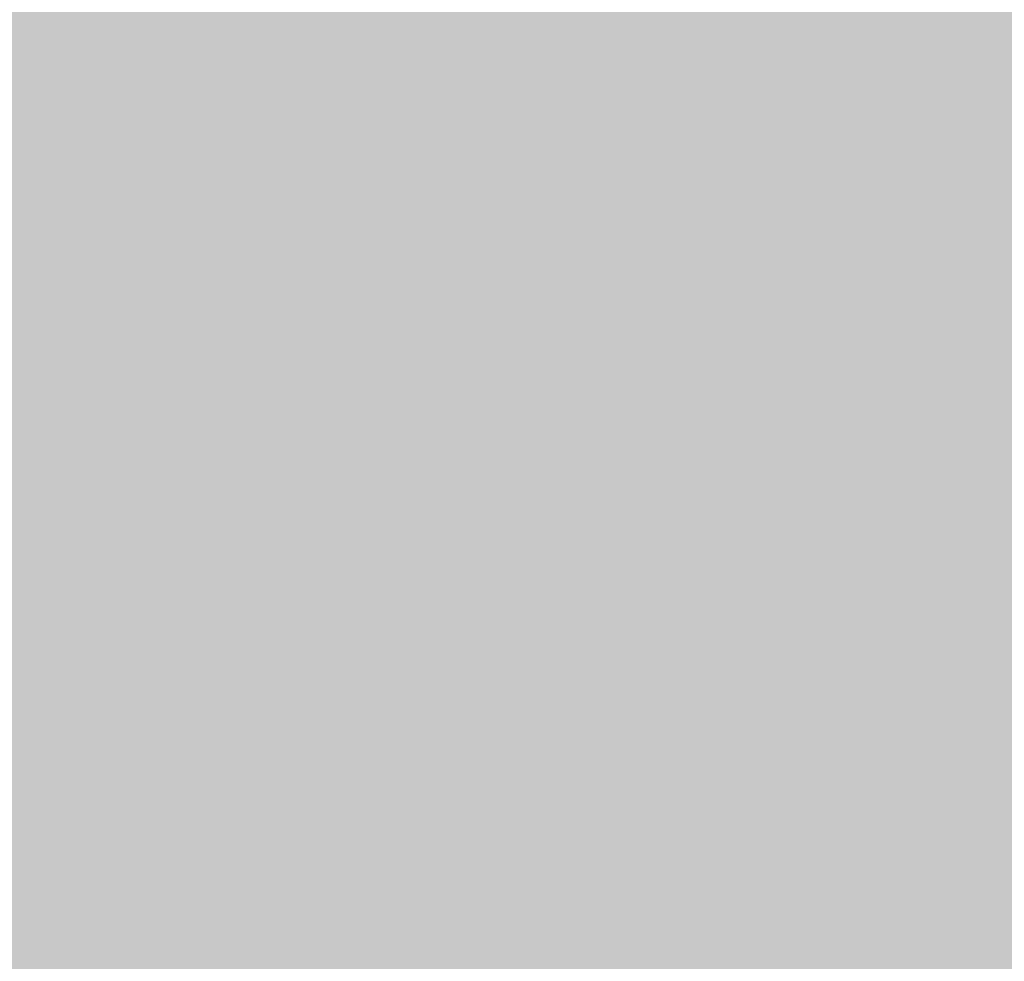
# Model space of a CAD drawing. Units: millimetres. Extents: x 0 to 2267, y 0 to 1823.
# Tile 202 of 256: x 1838.83 to 1841.442, y 1129.649 to 1132.147. Entities that reach past the tile are written whole.
import ezdxf

# ---------------------------------------------------------------- set-up
doc = ezdxf.new("R2010")
doc.units = ezdxf.units.MM
doc.header["$MEASUREMENT"] = 0
doc.layers.add('M-HATC', color=252, linetype='Continuous', lineweight=18)

msp = doc.modelspace()

# ---------------------------------------------------------------- hatches: boundary and pattern name
at = {"layer": 'M-HATC'}
h = msp.add_hatch(color=256, dxfattribs=at)
h.dxf.hatch_style = 1
h.paths.add_polyline_path([(2055.771, 1603.062), (1381.0868, 1603.062), (1381.0868, 1598.062), (2055.771, 1598.062)])
h.paths.add_polyline_path([(2055.771, 1598.062), (1381.0868, 1598.062), (1381.0868, 1593.062), (2055.771, 1593.062)])
h.paths.add_polyline_path([(2051.3074, 1536.7609), (1385.5504, 1536.7609), (1385.5504, 1526.7609), (1387.5504, 1526.7609), (1388.5366, 1525.0528), (1385.3319, 1521.2335), (1385.3319, 1521.2226), (2050.2542, 1522.7491), (2048.3212, 1525.0528), (2049.3074, 1526.7609), (2051.3074, 1526.7609)])
edge = h.paths.add_edge_path()
edge.add_arc((1847.5345, 1379.1492), 135, 222.603061, 222.890851, ccw=False)
edge.add_line((1748.1663, 1287.7656), (1683.0921, 1287.7656))
edge.add_arc((1583.7239, 1379.1492), 135, 317.109149, 317.396939, ccw=False)
edge.add_arc((1678.9686, 1290.6707), 5, 222.8909, 317.1091, ccw=False)
edge.add_arc((1774.2133, 1379.1492), 135, 222.603061, 222.890851, ccw=False)
edge.add_line((1674.8451, 1287.7656), (1609.7709, 1287.7656))
edge.add_arc((1510.4027, 1379.1492), 135, 317.109149, 317.396939, ccw=False)
edge.add_arc((1605.6474, 1290.6707), 5, 222.8909, 317.1091, ccw=False)
edge.add_arc((1700.8921, 1379.1492), 135, 222.603061, 222.890851, ccw=False)
edge.add_line((1601.5239, 1287.7656), (1536.4497, 1287.7656))
edge.add_arc((1437.0815, 1379.1492), 135, 317.109149, 317.396939, ccw=False)
edge.add_arc((1532.3262, 1290.6707), 5, 222.8909, 317.1091, ccw=False)
edge.add_arc((1627.5709, 1379.1492), 135, 222.603061, 222.890851, ccw=False)
edge.add_line((1528.2027, 1287.7656), (1505.9289, 1287.7656))
edge.add_spline(control_points=[(1505.9289, 1287.7656), (1504.2622, 1287.7656), (1504.2622, 1282.7656), (1505.9289, 1282.7656)], knot_values=[0, 0, 0, 0, 5, 5, 5, 5], degree=3, periodic=0)
edge.add_line((1505.9289, 1282.7656), (1930.9289, 1282.7656))
edge.add_spline(control_points=[(1930.9289, 1282.7656), (1932.5956, 1282.7656), (1932.5956, 1287.7656), (1930.9289, 1287.7656)], knot_values=[0, 0, 0, 0, 5, 5, 5, 5], degree=3, periodic=0)
edge.add_line((1930.9289, 1287.7656), (1903.0557, 1287.7656))
edge.add_arc((1803.6875, 1379.1492), 135, 317.109149, 317.396939, ccw=False)
edge.add_arc((1898.9322, 1290.6707), 5, 222.8909, 317.1091, ccw=False)
edge.add_arc((1994.1769, 1379.1492), 135, 222.603061, 222.890851, ccw=False)
edge.add_line((1894.8087, 1287.7656), (1829.7345, 1287.7656))
edge.add_arc((1730.3663, 1379.1492), 135, 317.109149, 317.396939, ccw=False)
edge.add_arc((1825.611, 1290.6707), 5, 222.8909, 317.1091, ccw=False)
edge.add_arc((1920.8557, 1379.1492), 135, 222.603061, 222.890851, ccw=False)
edge.add_line((1821.4875, 1287.7656), (1756.4133, 1287.7656))
edge.add_arc((1657.0451, 1379.1492), 135, 317.109149, 317.396939, ccw=False)
edge.add_arc((1752.2898, 1290.6707), 5, 222.8909, 317.1091, ccw=False)
edge = h.paths.add_edge_path()
edge.add_spline(control_points=[(1843.4289, 1227.2475), (1845.0956, 1227.2475), (1845.0956, 1232.2475), (1843.4289, 1232.2475)], knot_values=[0, 0, 0, 0, 5, 5, 5, 5], degree=3, periodic=0)
edge.add_line((1843.4289, 1232.2475), (1593.4289, 1232.2475))
edge.add_spline(control_points=[(1593.4289, 1232.2475), (1591.7622, 1232.2475), (1591.7622, 1227.2475), (1593.4289, 1227.2475)], knot_values=[0, 0, 0, 0, 5, 5, 5, 5], degree=3, periodic=0)
edge.add_line((1593.4289, 1227.2475), (1843.4289, 1227.2475))
h.paths.add_polyline_path([(1905.9289, 1127.4171), (1530.9289, 1127.4171, 0.414214), (1520.9289, 1117.4171), (1530.9289, 1117.4171), (1915.9289, 1117.4171, 0.414214)])
edge = h.paths.add_edge_path()
edge.add_arc((1397.0858, 1498.4078), 12.7299, 90.78215, 190.87871, ccw=False)
edge.add_line((1396.912, 1511.1365), (1428.0097, 1511.3488))
edge.add_line((1428.0097, 1511.3488), (1433.0097, 1511.3488))
edge.add_line((1433.0097, 1511.3488), (1434.439, 1511.3488))
edge.add_arc((1419.474, 1498.0804), 20, 41.561, 74.08211)
edge.add_line((1424.9592, 1517.3135), (1399.9351, 1517.2561))
edge.add_spline(control_points=[(1399.9307, 1517.2561), (1399.884, 1517.2131), (1399.8328, 1517.1689), (1399.7774, 1517.1236)], knot_values=[11.567499, 11.567499, 11.567499, 11.567499, 11.814249, 11.814249, 11.814249, 11.814249], degree=3, periodic=0)
edge.add_spline(control_points=[(1399.6328, 1517.0099), (1399.5831, 1516.9721), (1399.5307, 1516.9338), (1399.4759, 1516.8947)], knot_values=[11.167718, 11.167718, 11.167718, 11.167718, 11.365188, 11.365188, 11.365188, 11.365188], degree=3, periodic=0)
edge.add_spline(control_points=[(1399.3398, 1516.8001), (1399.1514, 1516.6719), (1398.9384, 1516.5377), (1398.704, 1516.3994)], knot_values=[10.376405, 10.376405, 10.376405, 10.376405, 11.00994, 11.00994, 11.00994, 11.00994], degree=3, periodic=0)
edge.add_spline(control_points=[(1398.6572, 1516.3719), (1398.5789, 1516.326), (1398.4983, 1516.2797), (1398.4155, 1516.2331)], knot_values=[10.125175, 10.125175, 10.125175, 10.125175, 10.334406, 10.334406, 10.334406, 10.334406], degree=3, periodic=0)
edge.add_spline(control_points=[(1398.2642, 1516.1487), (1398.196, 1516.1111), (1398.1263, 1516.0732), (1398.0555, 1516.0351)], knot_values=[9.832246, 9.832246, 9.832246, 9.832246, 9.999658, 9.999658, 9.999658, 9.999658], degree=3, periodic=0)
edge.add_spline(control_points=[(1397.9987, 1516.0048), (1397.7312, 1515.8621), (1397.446, 1515.7171), (1397.1466, 1515.5714)], knot_values=[9.161808, 9.161808, 9.161808, 9.161808, 9.787769, 9.787769, 9.787769, 9.787769], degree=3, periodic=0)
edge.add_spline(control_points=[(1397.1466, 1515.5714), (1396.8418, 1515.423), (1396.5222, 1515.274), (1396.1914, 1515.1262)], knot_values=[8.524455, 8.524455, 8.524455, 8.524455, 9.161808, 9.161808, 9.161808, 9.161808], degree=3, periodic=0)
edge.add_spline(control_points=[(1396.0777, 1515.0756), (1395.9854, 1515.0348), (1395.8922, 1514.994), (1395.7983, 1514.9534)], knot_values=[8.275193, 8.275193, 8.275193, 8.275193, 8.451726, 8.451726, 8.451726, 8.451726], degree=3, periodic=0)
edge.add_spline(control_points=[(1395.6018, 1514.8691), (1395.4997, 1514.8257), (1395.3968, 1514.7824), (1395.2932, 1514.7394)], knot_values=[7.962917, 7.962917, 7.962917, 7.962917, 8.152764, 8.152764, 8.152764, 8.152764], degree=3, periodic=0)
edge.add_spline(control_points=[(1395.2116, 1514.7057), (1394.8278, 1514.5475), (1394.4345, 1514.3929), (1394.0364, 1514.2442)], knot_values=[7.21254, 7.21254, 7.21254, 7.21254, 7.913148, 7.913148, 7.913148, 7.913148], degree=3, periodic=0)
edge.add_spline(control_points=[(1394.0364, 1514.2442), (1393.7076, 1514.1214), (1393.3754, 1514.0027), (1393.0427, 1513.8895)], knot_values=[6.633733, 6.633733, 6.633733, 6.633733, 7.21254, 7.21254, 7.21254, 7.21254], degree=3, periodic=0)
edge.add_spline(control_points=[(1392.8214, 1513.815), (1392.7198, 1513.7812), (1392.6181, 1513.7479), (1392.5166, 1513.7152)], knot_values=[6.328796, 6.328796, 6.328796, 6.328796, 6.505493, 6.505493, 6.505493, 6.505493], degree=3, periodic=0)
edge.add_spline(control_points=[(1392.5166, 1513.7152), (1392.3187, 1513.6515), (1392.1212, 1513.59), (1391.9244, 1513.531)], knot_values=[5.984605, 5.984605, 5.984605, 5.984605, 6.328796, 6.328796, 6.328796, 6.328796], degree=3, periodic=0)
edge.add_spline(control_points=[(1391.7915, 1513.4915), (1391.3122, 1513.3501), (1390.8384, 1513.2239), (1390.3784, 1513.1171)], knot_values=[5.066697, 5.066697, 5.066697, 5.066697, 5.907055, 5.907055, 5.907055, 5.907055], degree=3, periodic=0)
edge.add_spline(control_points=[(1390.3784, 1513.1171), (1390.1797, 1513.071), (1389.9836, 1513.0284), (1389.7907, 1512.9899)], knot_values=[4.70367, 4.70367, 4.70367, 4.70367, 5.066695, 5.066695, 5.066695, 5.066695], degree=3, periodic=0)
edge.add_spline(control_points=[(1389.422, 1512.9204), (1389.2459, 1512.8892), (1389.0729, 1512.8617), (1388.9036, 1512.8381)], knot_values=[4.130571, 4.130571, 4.130571, 4.130571, 4.469816, 4.469816, 4.469816, 4.469816], degree=3, periodic=0)
edge.add_spline(control_points=[(1388.9036, 1512.8381), (1388.591, 1512.7946), (1388.2911, 1512.7644), (1388.0071, 1512.7494)], knot_values=[3.504031, 3.504031, 3.504031, 3.504031, 4.130571, 4.130571, 4.130571, 4.130571], degree=3, periodic=0)
edge.add_spline(control_points=[(1387.9356, 1512.7459), (1387.8538, 1512.7423), (1387.7733, 1512.74), (1387.6944, 1512.739)], knot_values=[3.268866, 3.268866, 3.268866, 3.268866, 3.451164, 3.451164, 3.451164, 3.451164], degree=3, periodic=0)
edge.add_spline(control_points=[(1387.3351, 1512.7443), (1387.2076, 1512.7499), (1387.0847, 1512.7597), (1386.967, 1512.7739)], knot_values=[2.670686, 2.670686, 2.670686, 2.670686, 2.984, 2.984, 2.984, 2.984], degree=3, periodic=0)
edge.add_spline(control_points=[(1386.8327, 1512.7922), (1386.8209, 1512.7941), (1386.8092, 1512.7959), (1386.7975, 1512.7979)], knot_values=[2.516981, 2.516981, 2.516981, 2.516981, 2.549528, 2.549528, 2.549528, 2.549528], degree=3, periodic=0)
edge.add_spline(control_points=[(1386.4526, 1512.8735), (1386.4257, 1512.881), (1386.3993, 1512.889), (1386.3733, 1512.8972)], knot_values=[2.095869, 2.095869, 2.095869, 2.095869, 2.17941, 2.17941, 2.17941, 2.17941], degree=3, periodic=0)
edge.add_spline(control_points=[(1386.0691, 1513.0189), (1386.0634, 1513.0217), (1386.0577, 1513.0246), (1386.052, 1513.0275)], knot_values=[1.72453, 1.72453, 1.72453, 1.72453, 1.745933, 1.745933, 1.745933, 1.745933], degree=3, periodic=0)
edge.add_arc((1399.474, 1498.0804), 20, 131.82432, 180)
edge.add_arc((1630.3336, 1505.5484), 250.9708, 181.705176, 236.427975)
edge.add_arc((1605.3399, 1483.3044), 218.7822, 238.660829, 243.34961)
edge.add_arc((1647.0911, 1510.3592), 262.8986, 183.129836, 237.853442, ccw=False)
h.paths.add_polyline_path([(1406.5369, 1391.9644, 0.149382), (1491.5506, 1296.4418, -0.129517)], flags=17)
edge = h.paths.add_edge_path()
edge.add_arc((2037.3838, 1498.0804), 20, 0, 48.26587)
edge.add_spline(control_points=[(2050.6973, 1513.0052), (2050.6512, 1512.9847), (2050.6034, 1512.9655), (2050.5539, 1512.9477)], knot_values=[1.835652, 1.835652, 1.835652, 1.835652, 2.000781, 2.000781, 2.000781, 2.000781], degree=3, periodic=0)
edge.add_spline(control_points=[(2050.4616, 1512.9166), (2050.479, 1512.9221), (2050.4963, 1512.9277), (2050.5133, 1512.9335)], knot_values=[2.045477, 2.045477, 2.045477, 2.045477, 2.101389, 2.101389, 2.101389, 2.101389], degree=3, periodic=0)
edge.add_spline(control_points=[(2050.129, 1512.8342), (2050.1984, 1512.8473), (2050.2657, 1512.8623), (2050.3308, 1512.8792)], knot_values=[2.237629, 2.237629, 2.237629, 2.237629, 2.435841, 2.435841, 2.435841, 2.435841], degree=3, periodic=0)
edge.add_spline(control_points=[(2050.0946, 1512.8278), (2050.1061, 1512.8299), (2050.1176, 1512.832), (2050.129, 1512.8342)], knot_values=[2.435841, 2.435841, 2.435841, 2.435841, 2.468321, 2.468321, 2.468321, 2.468321], degree=3, periodic=0)
edge.add_spline(control_points=[(2049.7843, 1512.7851), (2049.8552, 1512.7922), (2049.9243, 1512.8008), (2049.9917, 1512.8109)], knot_values=[2.563852, 2.563852, 2.563852, 2.563852, 2.748541, 2.748541, 2.748541, 2.748541], degree=3, periodic=0)
edge.add_spline(control_points=[(2049.4052, 1512.7617), (2049.5364, 1512.7653), (2049.6629, 1512.773), (2049.7843, 1512.7851)], knot_values=[2.748541, 2.748541, 2.748541, 2.748541, 3.064882, 3.064882, 3.064882, 3.064882], degree=3, periodic=0)
edge.add_spline(control_points=[(2049.1698, 1512.7597), (2049.2336, 1512.7591), (2049.2965, 1512.7594), (2049.3584, 1512.7606)], knot_values=[3.102309, 3.102309, 3.102309, 3.102309, 3.2503, 3.2503, 3.2503, 3.2503], degree=3, periodic=0)
edge.add_spline(control_points=[(2048.8573, 1512.7691), (2048.9638, 1512.7638), (2049.068, 1512.7606), (2049.1698, 1512.7597)], knot_values=[3.2503, 3.2503, 3.2503, 3.2503, 3.486069, 3.486069, 3.486069, 3.486069], degree=3, periodic=0)
edge.add_spline(control_points=[(2048.6924, 1512.7789), (2048.3729, 1512.8009), (2048.0345, 1512.8411), (2047.6817, 1512.897)], knot_values=[3.606429, 3.606429, 3.606429, 3.606429, 4.2989, 4.2989, 4.2989, 4.2989], degree=3, periodic=0)
edge.add_spline(control_points=[(2047.6817, 1512.897), (2047.5458, 1512.9185), (2047.4077, 1512.9424), (2047.2678, 1512.9685)], knot_values=[4.2989, 4.2989, 4.2989, 4.2989, 4.565769, 4.565769, 4.565769, 4.565769], degree=3, periodic=0)
edge.add_spline(control_points=[(2047.2678, 1512.9685), (2047.1449, 1512.9914), (2047.0207, 1513.016), (2046.8951, 1513.0422)], knot_values=[4.565769, 4.565769, 4.565769, 4.565769, 4.799971, 4.799971, 4.799971, 4.799971], degree=3, periodic=0)
edge.add_spline(control_points=[(2046.8951, 1513.0422), (2046.5286, 1513.1188), (2046.1513, 1513.209), (2045.7676, 1513.3107)], knot_values=[4.799971, 4.799971, 4.799971, 4.799971, 5.483718, 5.483718, 5.483718, 5.483718], degree=3, periodic=0)
edge.add_spline(control_points=[(2045.7676, 1513.3107), (2045.3724, 1513.4154), (2044.9704, 1513.5322), (2044.5662, 1513.6588)], knot_values=[5.483718, 5.483718, 5.483718, 5.483718, 6.187866, 6.187866, 6.187866, 6.187866], degree=3, periodic=0)
edge.add_spline(control_points=[(2044.5662, 1513.6588), (2044.4149, 1513.7061), (2044.2633, 1513.7549), (2044.1116, 1513.8048)], knot_values=[6.187866, 6.187866, 6.187866, 6.187866, 6.451551, 6.451551, 6.451551, 6.451551], degree=3, periodic=0)
edge.add_spline(control_points=[(2044.1116, 1513.8048), (2043.9967, 1513.8427), (2043.8817, 1513.8813), (2043.7668, 1513.9205)], knot_values=[6.451551, 6.451551, 6.451551, 6.451551, 6.651434, 6.651434, 6.651434, 6.651434], degree=3, periodic=0)
edge.add_spline(control_points=[(2043.7668, 1513.9205), (2043.3716, 1514.0554), (2042.9774, 1514.1979), (2042.5886, 1514.3458)], knot_values=[6.651434, 6.651434, 6.651434, 6.651434, 7.338879, 7.338879, 7.338879, 7.338879], degree=3, periodic=0)
edge.add_spline(control_points=[(2042.5886, 1514.3458), (2042.1643, 1514.5071), (2041.7465, 1514.6749), (2041.3409, 1514.846)], knot_values=[7.338879, 7.338879, 7.338879, 7.338879, 8.089209, 8.089209, 8.089209, 8.089209], degree=3, periodic=0)
edge.add_spline(control_points=[(2041.3409, 1514.846), (2041.1028, 1514.9465), (2040.869, 1515.0481), (2040.6405, 1515.1502)], knot_values=[8.089209, 8.089209, 8.089209, 8.089209, 8.529587, 8.529587, 8.529587, 8.529587], degree=3, periodic=0)
edge.add_spline(control_points=[(2040.51, 1515.2089), (2040.0824, 1515.4022), (2039.6747, 1515.5971), (2039.295, 1515.7894)], knot_values=[8.613818, 8.613818, 8.613818, 8.613818, 9.44571, 9.44571, 9.44571, 9.44571], degree=3, periodic=0)
edge.add_spline(control_points=[(2039.295, 1515.7894), (2039.0618, 1515.9075), (2038.8391, 1516.0246), (2038.6288, 1516.1398)], knot_values=[9.44571, 9.44571, 9.44571, 9.44571, 9.956404, 9.956404, 9.956404, 9.956404], degree=3, periodic=0)
edge.add_spline(control_points=[(2038.6288, 1516.1398), (2038.5187, 1516.2001), (2038.4121, 1516.2598), (2038.309, 1516.3189)], knot_values=[9.956404, 9.956404, 9.956404, 9.956404, 10.223542, 10.223542, 10.223542, 10.223542], degree=3, periodic=0)
edge.add_spline(control_points=[(2038.309, 1516.3189), (2038.2138, 1516.3735), (2038.1216, 1516.4276), (2038.0328, 1516.481)], knot_values=[10.223542, 10.223542, 10.223542, 10.223542, 10.47051, 10.47051, 10.47051, 10.47051], degree=3, periodic=0)
edge.add_spline(control_points=[(2038.0328, 1516.481), (2037.7855, 1516.6296), (2037.5639, 1516.773), (2037.3722, 1516.909)], knot_values=[10.47051, 10.47051, 10.47051, 10.47051, 11.15767, 11.15767, 11.15767, 11.15767], degree=3, periodic=0)
edge.add_spline(control_points=[(2037.3722, 1516.909), (2037.2789, 1516.9752), (2037.1927, 1517.0396), (2037.1142, 1517.102)], knot_values=[11.15767, 11.15767, 11.15767, 11.15767, 11.49227, 11.49227, 11.49227, 11.49227], degree=3, periodic=0)
edge.add_spline(control_points=[(2036.8564, 1517.3259), (2036.9148, 1517.2692), (2036.9814, 1517.2103), (2037.0557, 1517.1492)], knot_values=[11.577341, 11.577341, 11.577341, 11.577341, 11.91035, 11.91035, 11.91035, 11.91035], degree=3, periodic=0)
edge.add_spline(control_points=[(2036.8074, 1517.3748), (2036.823, 1517.3587), (2036.8393, 1517.3424), (2036.8564, 1517.3259)], knot_values=[11.91035, 11.91035, 11.91035, 11.91035, 12.007402, 12.007402, 12.007402, 12.007402], degree=3, periodic=0)
edge.add_spline(control_points=[(2036.7017, 1517.494), (2036.7104, 1517.483), (2036.7196, 1517.4719), (2036.7291, 1517.4606)], knot_values=[12.184155, 12.184155, 12.184155, 12.184155, 12.255409, 12.255409, 12.255409, 12.255409], degree=3, periodic=0)
edge.add_spline(control_points=[(2036.6159, 1517.6205), (2036.62, 1517.613), (2036.6243, 1517.6055), (2036.6289, 1517.5979)], knot_values=[12.487913, 12.487913, 12.487913, 12.487913, 12.541035, 12.541035, 12.541035, 12.541035], degree=3, periodic=0)
edge.add_spline(control_points=[(2036.5635, 1517.786), (2036.5637, 1517.7794), (2036.5642, 1517.7726), (2036.565, 1517.7658)], knot_values=[12.911761, 12.911761, 12.911761, 12.911761, 12.968286, 12.968286, 12.968286, 12.968286], degree=3, periodic=0)
edge.add_spline(control_points=[(2036.6166, 1517.9304), (2036.6125, 1517.9259), (2036.6086, 1517.9212), (2036.6049, 1517.9165)], knot_values=[13.382527, 13.382527, 13.382527, 13.382527, 13.433791, 13.433791, 13.433791, 13.433791], degree=3, periodic=0)
edge.add_spline(control_points=[(2036.749, 1518.017), (2036.7361, 1518.0116), (2036.7239, 1518.006), (2036.7124, 1518.0002)], knot_values=[13.726299, 13.726299, 13.726299, 13.726299, 13.809928, 13.809928, 13.809928, 13.809928], degree=3, periodic=0)
edge.add_spline(control_points=[(2036.8604, 1518.0528), (2036.8386, 1518.0474), (2036.8181, 1518.0416), (2036.7988, 1518.0353)], knot_values=[13.910887, 13.910887, 13.910887, 13.910887, 14.02153, 14.02153, 14.02153, 14.02153], degree=3, periodic=0)
edge.add_line((2036.9639, 1518.0804), (2032.3838, 1518.0804))
edge.add_line((2032.3838, 1518.0804), (2027.3838, 1518.0804))
edge.add_line((2027.3838, 1518.0804), (2022.3838, 1518.0804))
edge.add_line((2022.3838, 1518.0804), (2017.3838, 1518.0804))
edge.add_arc((2017.3838, 1498.0804), 20, 90, 138.439)
edge.add_line((2002.4188, 1511.3488), (2003.8481, 1511.3488))
edge.add_line((2003.8481, 1511.3488), (2008.8481, 1511.3488))
edge.add_line((2008.8481, 1511.3488), (2039.772, 1511.1377))
edge.add_arc((2039.772, 1498.4078), 12.7299, -10.87871, 90, ccw=False)
edge.add_arc((1789.7668, 1510.3592), 262.8986, 302.146558, 356.870164, ccw=False)
edge.add_arc((1831.5179, 1483.3044), 218.7822, 296.65039, 301.339171)
edge.add_arc((1806.5242, 1505.5484), 250.9708, 303.572025, 358.294824)
h.paths.add_polyline_path([(2030.321, 1391.9644, -0.129517), (1945.3072, 1296.4418, 0.149382)], flags=17)
edge = h.paths.add_edge_path()
edge.add_spline(control_points=[(2037.2464, 1518.0821), (2037.2898, 1518.081), (2037.3355, 1518.0804), (2037.3838, 1518.0804)], knot_values=[0.000012, 0.000012, 0.000012, 0.000012, 0.144754, 0.144754, 0.144754, 0.144754], degree=3, periodic=0)
edge.add_line((2037.3357, 1518.0804), (2037.0096, 1518.0804))
edge.add_spline(control_points=[(2037.0096, 1518.0804), (2036.9822, 1518.0768), (2036.956, 1518.0727), (2036.9312, 1518.0681)], knot_values=[14.13465, 14.13465, 14.13465, 14.13465, 14.247197, 14.247197, 14.247197, 14.247197], degree=3, periodic=0)
edge.add_spline(control_points=[(2036.9312, 1518.0681), (2036.9276, 1518.0674), (2036.9241, 1518.0667), (2036.9205, 1518.0661)], knot_values=[14.118315, 14.118315, 14.118315, 14.118315, 14.13465, 14.13465, 14.13465, 14.13465], degree=3, periodic=0)
edge.add_spline(control_points=[(2036.9205, 1518.0661), (2036.9118, 1518.0644), (2036.9032, 1518.0626), (2036.8948, 1518.0608)], knot_values=[14.078086, 14.078086, 14.078086, 14.078086, 14.118315, 14.118315, 14.118315, 14.118315], degree=3, periodic=0)
edge.add_spline(control_points=[(2036.8948, 1518.0608), (2036.883, 1518.0583), (2036.8716, 1518.0556), (2036.8604, 1518.0528)], knot_values=[14.02153, 14.02153, 14.02153, 14.02153, 14.078086, 14.078086, 14.078086, 14.078086], degree=3, periodic=0)
edge.add_spline(control_points=[(2036.8604, 1518.0528), (2036.8386, 1518.0474), (2036.8181, 1518.0416), (2036.7988, 1518.0353)], knot_values=[13.910887, 13.910887, 13.910887, 13.910887, 14.02153, 14.02153, 14.02153, 14.02153], degree=3, periodic=0)
edge.add_spline(control_points=[(2036.7988, 1518.0353), (2036.7981, 1518.035), (2036.7974, 1518.0348), (2036.7967, 1518.0346)], knot_values=[13.906906, 13.906906, 13.906906, 13.906906, 13.910887, 13.910887, 13.910887, 13.910887], degree=3, periodic=0)
edge.add_spline(control_points=[(2036.7967, 1518.0346), (2036.7882, 1518.0318), (2036.7799, 1518.0289), (2036.7719, 1518.0259)], knot_values=[13.857826, 13.857826, 13.857826, 13.857826, 13.906906, 13.906906, 13.906906, 13.906906], degree=3, periodic=0)
edge.add_spline(control_points=[(2036.7719, 1518.0259), (2036.764, 1518.023), (2036.7564, 1518.02), (2036.749, 1518.017)], knot_values=[13.809928, 13.809928, 13.809928, 13.809928, 13.857826, 13.857826, 13.857826, 13.857826], degree=3, periodic=0)
edge.add_spline(control_points=[(2036.749, 1518.017), (2036.7361, 1518.0116), (2036.7239, 1518.006), (2036.7124, 1518.0002)], knot_values=[13.726299, 13.726299, 13.726299, 13.726299, 13.809928, 13.809928, 13.809928, 13.809928], degree=3, periodic=0)
edge.add_spline(control_points=[(2036.7124, 1518.0002), (2036.7121, 1518), (2036.7118, 1517.9999), (2036.7115, 1517.9997)], knot_values=[13.723993, 13.723993, 13.723993, 13.723993, 13.726299, 13.726299, 13.726299, 13.726299], degree=3, periodic=0)
edge.add_spline(control_points=[(2036.7115, 1517.9997), (2036.7063, 1517.9971), (2036.7013, 1517.9944), (2036.6965, 1517.9917)], knot_values=[13.686536, 13.686536, 13.686536, 13.686536, 13.723993, 13.723993, 13.723993, 13.723993], degree=3, periodic=0)
edge.add_spline(control_points=[(2036.6965, 1517.9917), (2036.6919, 1517.9891), (2036.6874, 1517.9865), (2036.6831, 1517.9839)], knot_values=[13.651251, 13.651251, 13.651251, 13.651251, 13.686536, 13.686536, 13.686536, 13.686536], degree=3, periodic=0)
edge.add_spline(control_points=[(2036.6831, 1517.9839), (2036.6764, 1517.9798), (2036.67, 1517.9757), (2036.6639, 1517.9714)], knot_values=[13.596804, 13.596804, 13.596804, 13.596804, 13.651251, 13.651251, 13.651251, 13.651251], degree=3, periodic=0)
edge.add_spline(control_points=[(2036.6639, 1517.9714), (2036.6636, 1517.9712), (2036.6633, 1517.9709), (2036.6629, 1517.9707)], knot_values=[13.593956, 13.593956, 13.593956, 13.593956, 13.596804, 13.596804, 13.596804, 13.596804], degree=3, periodic=0)
edge.add_spline(control_points=[(2036.6629, 1517.9707), (2036.6603, 1517.9689), (2036.6577, 1517.967), (2036.6552, 1517.9651)], knot_values=[13.570322, 13.570322, 13.570322, 13.570322, 13.593956, 13.593956, 13.593956, 13.593956], degree=3, periodic=0)
edge.add_spline(control_points=[(2036.6552, 1517.9651), (2036.6525, 1517.9631), (2036.6499, 1517.9611), (2036.6474, 1517.9591)], knot_values=[13.545477, 13.545477, 13.545477, 13.545477, 13.570322, 13.570322, 13.570322, 13.570322], degree=3, periodic=0)
edge.add_spline(control_points=[(2036.6474, 1517.9591), (2036.6472, 1517.9589), (2036.6471, 1517.9588), (2036.6469, 1517.9587)], knot_values=[13.543931, 13.543931, 13.543931, 13.543931, 13.545477, 13.545477, 13.545477, 13.545477], degree=3, periodic=0)
edge.add_spline(control_points=[(2036.6469, 1517.9587), (2036.6412, 1517.9541), (2036.6358, 1517.9494), (2036.6307, 1517.9447)], knot_values=[13.488237, 13.488237, 13.488237, 13.488237, 13.543931, 13.543931, 13.543931, 13.543931], degree=3, periodic=0)
edge.add_spline(control_points=[(2036.6307, 1517.9447), (2036.6282, 1517.9423), (2036.6257, 1517.9399), (2036.6233, 1517.9374)], knot_values=[13.460307, 13.460307, 13.460307, 13.460307, 13.488237, 13.488237, 13.488237, 13.488237], degree=3, periodic=0)
edge.add_spline(control_points=[(2036.6233, 1517.9374), (2036.6215, 1517.9356), (2036.6198, 1517.9338), (2036.6181, 1517.932)], knot_values=[13.439712, 13.439712, 13.439712, 13.439712, 13.460307, 13.460307, 13.460307, 13.460307], degree=3, periodic=0)
edge.add_spline(control_points=[(2036.6181, 1517.932), (2036.6176, 1517.9315), (2036.6171, 1517.9309), (2036.6166, 1517.9304)], knot_values=[13.433791, 13.433791, 13.433791, 13.433791, 13.439712, 13.439712, 13.439712, 13.439712], degree=3, periodic=0)
edge.add_spline(control_points=[(2036.6166, 1517.9304), (2036.6125, 1517.9259), (2036.6086, 1517.9212), (2036.6049, 1517.9165)], knot_values=[13.382527, 13.382527, 13.382527, 13.382527, 13.433791, 13.433791, 13.433791, 13.433791], degree=3, periodic=0)
edge.add_spline(control_points=[(2036.6049, 1517.9165), (2036.6026, 1517.9135), (2036.6004, 1517.9104), (2036.5982, 1517.9074)], knot_values=[13.350017, 13.350017, 13.350017, 13.350017, 13.382527, 13.382527, 13.382527, 13.382527], degree=3, periodic=0)
edge.add_spline(control_points=[(2036.5982, 1517.9074), (2036.5972, 1517.9059), (2036.5962, 1517.9043), (2036.5952, 1517.9028)], knot_values=[13.333922, 13.333922, 13.333922, 13.333922, 13.350017, 13.350017, 13.350017, 13.350017], degree=3, periodic=0)
edge.add_spline(control_points=[(2036.5952, 1517.9028), (2036.5945, 1517.9018), (2036.5939, 1517.9009), (2036.5933, 1517.8999)], knot_values=[13.323828, 13.323828, 13.323828, 13.323828, 13.333922, 13.333922, 13.333922, 13.333922], degree=3, periodic=0)
edge.add_spline(control_points=[(2036.5933, 1517.8999), (2036.5905, 1517.8955), (2036.5879, 1517.8909), (2036.5855, 1517.8864)], knot_values=[13.277545, 13.277545, 13.277545, 13.277545, 13.323828, 13.323828, 13.323828, 13.323828], degree=3, periodic=0)
edge.add_spline(control_points=[(2036.5855, 1517.8864), (2036.5836, 1517.8827), (2036.5817, 1517.8789), (2036.5801, 1517.8751)], knot_values=[13.240119, 13.240119, 13.240119, 13.240119, 13.277545, 13.277545, 13.277545, 13.277545], degree=3, periodic=0)
edge.add_spline(control_points=[(2036.5801, 1517.8751), (2036.5795, 1517.8739), (2036.579, 1517.8727), (2036.5785, 1517.8715)], knot_values=[13.228211, 13.228211, 13.228211, 13.228211, 13.240119, 13.240119, 13.240119, 13.240119], degree=3, periodic=0)
edge.add_spline(control_points=[(2036.5785, 1517.8715), (2036.578, 1517.8702), (2036.5774, 1517.869), (2036.5769, 1517.8677)], knot_values=[13.215717, 13.215717, 13.215717, 13.215717, 13.228211, 13.228211, 13.228211, 13.228211], degree=3, periodic=0)
edge.add_spline(control_points=[(2036.5769, 1517.8677), (2036.5755, 1517.864), (2036.5741, 1517.8603), (2036.5729, 1517.8565)], knot_values=[13.179847, 13.179847, 13.179847, 13.179847, 13.215717, 13.215717, 13.215717, 13.215717], degree=3, periodic=0)
edge.add_spline(control_points=[(2036.5729, 1517.8565), (2036.5713, 1517.8515), (2036.5699, 1517.8464), (2036.5687, 1517.8413)], knot_values=[13.132017, 13.132017, 13.132017, 13.132017, 13.179847, 13.179847, 13.179847, 13.179847], degree=3, periodic=0)
edge.add_spline(control_points=[(2036.5687, 1517.8413), (2036.5684, 1517.8402), (2036.5682, 1517.8392), (2036.568, 1517.8382)], knot_values=[13.122482, 13.122482, 13.122482, 13.122482, 13.132017, 13.132017, 13.132017, 13.132017], degree=3, periodic=0)
edge.add_spline(control_points=[(2036.568, 1517.8382), (2036.5676, 1517.8363), (2036.5672, 1517.8345), (2036.5669, 1517.8327)], knot_values=[13.105592, 13.105592, 13.105592, 13.105592, 13.122482, 13.122482, 13.122482, 13.122482], degree=3, periodic=0)
edge.add_spline(control_points=[(2036.5669, 1517.8327), (2036.5662, 1517.8292), (2036.5657, 1517.8257), (2036.5652, 1517.8222)], knot_values=[13.074063, 13.074063, 13.074063, 13.074063, 13.105592, 13.105592, 13.105592, 13.105592], degree=3, periodic=0)
edge.add_spline(control_points=[(2036.5652, 1517.8222), (2036.5652, 1517.8222), (2036.5652, 1517.8222), (2036.5652, 1517.8222)], knot_values=[13.074043, 13.074043, 13.074043, 13.074043, 13.074063, 13.074063, 13.074063, 13.074063], degree=3, periodic=0)
edge.add_spline(control_points=[(2036.5652, 1517.8222), (2036.5644, 1517.8164), (2036.5639, 1517.8106), (2036.5636, 1517.8046)], knot_values=[13.021884, 13.021884, 13.021884, 13.021884, 13.074043, 13.074043, 13.074043, 13.074043], degree=3, periodic=0)
edge.add_spline(control_points=[(2036.5636, 1517.8046), (2036.5636, 1517.804), (2036.5636, 1517.8034), (2036.5635, 1517.8028)], knot_values=[13.01674, 13.01674, 13.01674, 13.01674, 13.021884, 13.021884, 13.021884, 13.021884], degree=3, periodic=0)
edge.add_spline(control_points=[(2036.5635, 1517.8028), (2036.5634, 1517.8005), (2036.5634, 1517.7982), (2036.5634, 1517.7958)], knot_values=[12.996438, 12.996438, 12.996438, 12.996438, 13.01674, 13.01674, 13.01674, 13.01674], degree=3, periodic=0)
edge.add_spline(control_points=[(2036.5634, 1517.7958), (2036.5633, 1517.7926), (2036.5634, 1517.7893), (2036.5635, 1517.786)], knot_values=[12.968286, 12.968286, 12.968286, 12.968286, 12.996438, 12.996438, 12.996438, 12.996438], degree=3, periodic=0)
edge.add_spline(control_points=[(2036.5635, 1517.786), (2036.5637, 1517.7794), (2036.5642, 1517.7726), (2036.565, 1517.7658)], knot_values=[12.911761, 12.911761, 12.911761, 12.911761, 12.968286, 12.968286, 12.968286, 12.968286], degree=3, periodic=0)
edge.add_spline(control_points=[(2036.565, 1517.7658), (2036.565, 1517.7657), (2036.565, 1517.7656), (2036.565, 1517.7656)], knot_values=[12.911017, 12.911017, 12.911017, 12.911017, 12.911761, 12.911761, 12.911761, 12.911761], degree=3, periodic=0)
edge.add_spline(control_points=[(2036.565, 1517.7656), (2036.5654, 1517.7625), (2036.5658, 1517.7593), (2036.5663, 1517.7562)], knot_values=[12.88528, 12.88528, 12.88528, 12.88528, 12.911017, 12.911017, 12.911017, 12.911017], degree=3, periodic=0)
edge.add_spline(control_points=[(2036.5663, 1517.7562), (2036.5667, 1517.7534), (2036.5672, 1517.7506), (2036.5677, 1517.7478)], knot_values=[12.862519, 12.862519, 12.862519, 12.862519, 12.88528, 12.88528, 12.88528, 12.88528], degree=3, periodic=0)
edge.add_spline(control_points=[(2036.5677, 1517.7478), (2036.5678, 1517.7474), (2036.5679, 1517.7469), (2036.568, 1517.7465)], knot_values=[12.858885, 12.858885, 12.858885, 12.858885, 12.862519, 12.862519, 12.862519, 12.862519], degree=3, periodic=0)
edge.add_spline(control_points=[(2036.568, 1517.7465), (2036.5692, 1517.7399), (2036.5707, 1517.7332), (2036.5724, 1517.7264)], knot_values=[12.8053, 12.8053, 12.8053, 12.8053, 12.858885, 12.858885, 12.858885, 12.858885], degree=3, periodic=0)
edge.add_spline(control_points=[(2036.5724, 1517.7264), (2036.5734, 1517.7226), (2036.5745, 1517.7187), (2036.5756, 1517.7149)], knot_values=[12.775176, 12.775176, 12.775176, 12.775176, 12.8053, 12.8053, 12.8053, 12.8053], degree=3, periodic=0)
edge.add_spline(control_points=[(2036.5756, 1517.7149), (2036.5763, 1517.7125), (2036.577, 1517.7102), (2036.5778, 1517.7078)], knot_values=[12.756759, 12.756759, 12.756759, 12.756759, 12.775176, 12.775176, 12.775176, 12.775176], degree=3, periodic=0)
edge.add_spline(control_points=[(2036.5778, 1517.7078), (2036.5781, 1517.7067), (2036.5784, 1517.7057), (2036.5787, 1517.7047)], knot_values=[12.748742, 12.748742, 12.748742, 12.748742, 12.756759, 12.756759, 12.756759, 12.756759], degree=3, periodic=0)
edge.add_spline(control_points=[(2036.5787, 1517.7047), (2036.5808, 1517.6983), (2036.5831, 1517.6919), (2036.5856, 1517.6854)], knot_values=[12.69959, 12.69959, 12.69959, 12.69959, 12.748742, 12.748742, 12.748742, 12.748742], degree=3, periodic=0)
edge.add_spline(control_points=[(2036.5856, 1517.6854), (2036.5876, 1517.68), (2036.5898, 1517.6746), (2036.5921, 1517.6692)], knot_values=[12.659038, 12.659038, 12.659038, 12.659038, 12.69959, 12.69959, 12.69959, 12.69959], degree=3, periodic=0)
edge.add_spline(control_points=[(2036.5921, 1517.6692), (2036.594, 1517.6648), (2036.5959, 1517.6605), (2036.5979, 1517.6561)], knot_values=[12.626806, 12.626806, 12.626806, 12.626806, 12.659038, 12.659038, 12.659038, 12.659038], degree=3, periodic=0)
edge.add_spline(control_points=[(2036.5979, 1517.6561), (2036.5984, 1517.6551), (2036.5989, 1517.6541), (2036.5993, 1517.6531)], knot_values=[12.619394, 12.619394, 12.619394, 12.619394, 12.626806, 12.626806, 12.626806, 12.626806], degree=3, periodic=0)
edge.add_spline(control_points=[(2036.5993, 1517.6531), (2036.6043, 1517.6424), (2036.6099, 1517.6315), (2036.6159, 1517.6205)], knot_values=[12.541039, 12.541039, 12.541039, 12.541039, 12.619394, 12.619394, 12.619394, 12.619394], degree=3, periodic=0)
edge.add_spline(control_points=[(2036.6159, 1517.6205), (2036.6159, 1517.6205), (2036.6159, 1517.6205), (2036.6159, 1517.6205)], knot_values=[12.541035, 12.541035, 12.541035, 12.541035, 12.541039, 12.541039, 12.541039, 12.541039], degree=3, periodic=0)
edge.add_spline(control_points=[(2036.6159, 1517.6205), (2036.62, 1517.613), (2036.6243, 1517.6055), (2036.6289, 1517.5979)], knot_values=[12.487913, 12.487913, 12.487913, 12.487913, 12.541035, 12.541035, 12.541035, 12.541035], degree=3, periodic=0)
edge.add_spline(control_points=[(2036.6289, 1517.5979), (2036.6326, 1517.5916), (2036.6365, 1517.5853), (2036.6406, 1517.5789)], knot_values=[12.443982, 12.443982, 12.443982, 12.443982, 12.487913, 12.487913, 12.487913, 12.487913], degree=3, periodic=0)
edge.add_spline(control_points=[(2036.6406, 1517.5789), (2036.6414, 1517.5776), (2036.6423, 1517.5763), (2036.6431, 1517.5749)], knot_values=[12.434996, 12.434996, 12.434996, 12.434996, 12.443982, 12.443982, 12.443982, 12.443982], degree=3, periodic=0)
edge.add_spline(control_points=[(2036.6431, 1517.5749), (2036.6531, 1517.5596), (2036.6639, 1517.5439), (2036.6756, 1517.528)], knot_values=[12.329647, 12.329647, 12.329647, 12.329647, 12.434996, 12.434996, 12.434996, 12.434996], degree=3, periodic=0)
edge.add_spline(control_points=[(2036.6756, 1517.528), (2036.6839, 1517.5168), (2036.6925, 1517.5055), (2036.7017, 1517.494)], knot_values=[12.255409, 12.255409, 12.255409, 12.255409, 12.329647, 12.329647, 12.329647, 12.329647], degree=3, periodic=0)
edge.add_spline(control_points=[(2036.7017, 1517.494), (2036.7104, 1517.483), (2036.7196, 1517.4719), (2036.7291, 1517.4606)], knot_values=[12.184155, 12.184155, 12.184155, 12.184155, 12.255409, 12.255409, 12.255409, 12.255409], degree=3, periodic=0)
edge.add_spline(control_points=[(2036.7291, 1517.4606), (2036.7436, 1517.4435), (2036.759, 1517.4262), (2036.7753, 1517.4085)], knot_values=[12.075961, 12.075961, 12.075961, 12.075961, 12.184155, 12.184155, 12.184155, 12.184155], degree=3, periodic=0)
edge.add_spline(control_points=[(2036.7753, 1517.4085), (2036.7763, 1517.4075), (2036.7773, 1517.4064), (2036.7783, 1517.4054)], knot_values=[12.069502, 12.069502, 12.069502, 12.069502, 12.075961, 12.075961, 12.075961, 12.075961], degree=3, periodic=0)
edge.add_spline(control_points=[(2036.7783, 1517.4054), (2036.7877, 1517.3953), (2036.7974, 1517.385), (2036.8074, 1517.3748)], knot_values=[12.007402, 12.007402, 12.007402, 12.007402, 12.069502, 12.069502, 12.069502, 12.069502], degree=3, periodic=0)
edge.add_spline(control_points=[(2036.8074, 1517.3748), (2036.823, 1517.3587), (2036.8393, 1517.3424), (2036.8564, 1517.3259)], knot_values=[11.91035, 11.91035, 11.91035, 11.91035, 12.007402, 12.007402, 12.007402, 12.007402], degree=3, periodic=0)
edge.add_spline(control_points=[(2036.8564, 1517.3259), (2036.9148, 1517.2692), (2036.9814, 1517.2103), (2037.0557, 1517.1492)], knot_values=[11.577341, 11.577341, 11.577341, 11.577341, 11.91035, 11.91035, 11.91035, 11.91035], degree=3, periodic=0)
edge.add_spline(control_points=[(2037.0557, 1517.1492), (2037.0747, 1517.1336), (2037.0942, 1517.1179), (2037.1142, 1517.102)], knot_values=[11.49227, 11.49227, 11.49227, 11.49227, 11.577341, 11.577341, 11.577341, 11.577341], degree=3, periodic=0)
edge.add_spline(control_points=[(2037.1142, 1517.102), (2037.1927, 1517.0396), (2037.2789, 1516.9752), (2037.3722, 1516.909)], knot_values=[11.15767, 11.15767, 11.15767, 11.15767, 11.49227, 11.49227, 11.49227, 11.49227], degree=3, periodic=0)
edge.add_spline(control_points=[(2037.3722, 1516.909), (2037.5639, 1516.773), (2037.7855, 1516.6296), (2038.0328, 1516.481)], knot_values=[10.47051, 10.47051, 10.47051, 10.47051, 11.15767, 11.15767, 11.15767, 11.15767], degree=3, periodic=0)
edge.add_spline(control_points=[(2038.0328, 1516.481), (2038.1216, 1516.4276), (2038.2138, 1516.3735), (2038.309, 1516.3189)], knot_values=[10.223542, 10.223542, 10.223542, 10.223542, 10.47051, 10.47051, 10.47051, 10.47051], degree=3, periodic=0)
edge.add_spline(control_points=[(2038.309, 1516.3189), (2038.4121, 1516.2598), (2038.5187, 1516.2001), (2038.6288, 1516.1398)], knot_values=[9.956404, 9.956404, 9.956404, 9.956404, 10.223542, 10.223542, 10.223542, 10.223542], degree=3, periodic=0)
edge.add_spline(control_points=[(2038.6288, 1516.1398), (2038.8391, 1516.0246), (2039.0618, 1515.9075), (2039.295, 1515.7894)], knot_values=[9.44571, 9.44571, 9.44571, 9.44571, 9.956404, 9.956404, 9.956404, 9.956404], degree=3, periodic=0)
edge.add_spline(control_points=[(2039.295, 1515.7894), (2039.6747, 1515.5971), (2040.0824, 1515.4022), (2040.51, 1515.2089)], knot_values=[8.613818, 8.613818, 8.613818, 8.613818, 9.44571, 9.44571, 9.44571, 9.44571], degree=3, periodic=0)
edge.add_spline(control_points=[(2040.51, 1515.2089), (2040.5533, 1515.1893), (2040.5968, 1515.1697), (2040.6405, 1515.1502)], knot_values=[8.529587, 8.529587, 8.529587, 8.529587, 8.613818, 8.613818, 8.613818, 8.613818], degree=3, periodic=0)
edge.add_spline(control_points=[(2040.6405, 1515.1502), (2040.869, 1515.0481), (2041.1028, 1514.9465), (2041.3409, 1514.846)], knot_values=[8.089209, 8.089209, 8.089209, 8.089209, 8.529587, 8.529587, 8.529587, 8.529587], degree=3, periodic=0)
edge.add_spline(control_points=[(2041.3409, 1514.846), (2041.7465, 1514.6749), (2042.1643, 1514.5071), (2042.5886, 1514.3458)], knot_values=[7.338879, 7.338879, 7.338879, 7.338879, 8.089209, 8.089209, 8.089209, 8.089209], degree=3, periodic=0)
edge.add_spline(control_points=[(2042.5886, 1514.3458), (2042.9774, 1514.1979), (2043.3716, 1514.0554), (2043.7668, 1513.9205)], knot_values=[6.651434, 6.651434, 6.651434, 6.651434, 7.338879, 7.338879, 7.338879, 7.338879], degree=3, periodic=0)
edge.add_spline(control_points=[(2043.7668, 1513.9205), (2043.8817, 1513.8813), (2043.9967, 1513.8427), (2044.1116, 1513.8048)], knot_values=[6.451551, 6.451551, 6.451551, 6.451551, 6.651434, 6.651434, 6.651434, 6.651434], degree=3, periodic=0)
edge.add_spline(control_points=[(2044.1116, 1513.8048), (2044.2633, 1513.7549), (2044.4149, 1513.7061), (2044.5662, 1513.6588)], knot_values=[6.187866, 6.187866, 6.187866, 6.187866, 6.451551, 6.451551, 6.451551, 6.451551], degree=3, periodic=0)
edge.add_spline(control_points=[(2044.5662, 1513.6588), (2044.9704, 1513.5322), (2045.3724, 1513.4154), (2045.7676, 1513.3107)], knot_values=[5.483718, 5.483718, 5.483718, 5.483718, 6.187866, 6.187866, 6.187866, 6.187866], degree=3, periodic=0)
edge.add_spline(control_points=[(2045.7676, 1513.3107), (2046.1513, 1513.209), (2046.5286, 1513.1188), (2046.8951, 1513.0422)], knot_values=[4.799971, 4.799971, 4.799971, 4.799971, 5.483718, 5.483718, 5.483718, 5.483718], degree=3, periodic=0)
edge.add_spline(control_points=[(2046.8951, 1513.0422), (2047.0207, 1513.016), (2047.1449, 1512.9914), (2047.2678, 1512.9685)], knot_values=[4.565769, 4.565769, 4.565769, 4.565769, 4.799971, 4.799971, 4.799971, 4.799971], degree=3, periodic=0)
edge.add_spline(control_points=[(2047.2678, 1512.9685), (2047.4077, 1512.9424), (2047.5458, 1512.9185), (2047.6817, 1512.897)], knot_values=[4.2989, 4.2989, 4.2989, 4.2989, 4.565769, 4.565769, 4.565769, 4.565769], degree=3, periodic=0)
edge.add_spline(control_points=[(2047.6817, 1512.897), (2048.0345, 1512.8411), (2048.3729, 1512.8009), (2048.6924, 1512.7789)], knot_values=[3.606429, 3.606429, 3.606429, 3.606429, 4.2989, 4.2989, 4.2989, 4.2989], degree=3, periodic=0)
edge.add_spline(control_points=[(2048.6924, 1512.7789), (2048.7479, 1512.7751), (2048.8029, 1512.7718), (2048.8573, 1512.7691)], knot_values=[3.486069, 3.486069, 3.486069, 3.486069, 3.606429, 3.606429, 3.606429, 3.606429], degree=3, periodic=0)
edge.add_spline(control_points=[(2048.8573, 1512.7691), (2048.9638, 1512.7638), (2049.068, 1512.7606), (2049.1698, 1512.7597)], knot_values=[3.2503, 3.2503, 3.2503, 3.2503, 3.486069, 3.486069, 3.486069, 3.486069], degree=3, periodic=0)
edge.add_spline(control_points=[(2049.1698, 1512.7597), (2049.2336, 1512.7591), (2049.2965, 1512.7594), (2049.3584, 1512.7606)], knot_values=[3.102309, 3.102309, 3.102309, 3.102309, 3.2503, 3.2503, 3.2503, 3.2503], degree=3, periodic=0)
edge.add_spline(control_points=[(2049.3584, 1512.7606), (2049.3741, 1512.7609), (2049.3897, 1512.7613), (2049.4052, 1512.7617)], knot_values=[3.064882, 3.064882, 3.064882, 3.064882, 3.102309, 3.102309, 3.102309, 3.102309], degree=3, periodic=0)
edge.add_spline(control_points=[(2049.4052, 1512.7617), (2049.5364, 1512.7653), (2049.6629, 1512.773), (2049.7843, 1512.7851)], knot_values=[2.748541, 2.748541, 2.748541, 2.748541, 3.064882, 3.064882, 3.064882, 3.064882], degree=3, periodic=0)
edge.add_spline(control_points=[(2049.7843, 1512.7851), (2049.8552, 1512.7922), (2049.9243, 1512.8008), (2049.9917, 1512.8109)], knot_values=[2.563852, 2.563852, 2.563852, 2.563852, 2.748541, 2.748541, 2.748541, 2.748541], degree=3, periodic=0)
edge.add_spline(control_points=[(2049.9917, 1512.8109), (2050.0265, 1512.8161), (2050.0608, 1512.8218), (2050.0946, 1512.8278)], knot_values=[2.468321, 2.468321, 2.468321, 2.468321, 2.563852, 2.563852, 2.563852, 2.563852], degree=3, periodic=0)
edge.add_spline(control_points=[(2050.0946, 1512.8278), (2050.1061, 1512.8299), (2050.1176, 1512.832), (2050.129, 1512.8342)], knot_values=[2.435841, 2.435841, 2.435841, 2.435841, 2.468321, 2.468321, 2.468321, 2.468321], degree=3, periodic=0)
edge.add_spline(control_points=[(2050.129, 1512.8342), (2050.1984, 1512.8473), (2050.2657, 1512.8623), (2050.3308, 1512.8792)], knot_values=[2.237629, 2.237629, 2.237629, 2.237629, 2.435841, 2.435841, 2.435841, 2.435841], degree=3, periodic=0)
edge.add_spline(control_points=[(2050.3308, 1512.8792), (2050.3754, 1512.8908), (2050.4191, 1512.9032), (2050.4616, 1512.9166)], knot_values=[2.101389, 2.101389, 2.101389, 2.101389, 2.237629, 2.237629, 2.237629, 2.237629], degree=3, periodic=0)
edge.add_spline(control_points=[(2050.4616, 1512.9166), (2050.479, 1512.9221), (2050.4963, 1512.9277), (2050.5133, 1512.9335)], knot_values=[2.045477, 2.045477, 2.045477, 2.045477, 2.101389, 2.101389, 2.101389, 2.101389], degree=3, periodic=0)
edge.add_spline(control_points=[(2050.5133, 1512.9335), (2050.527, 1512.9382), (2050.5405, 1512.9429), (2050.5539, 1512.9477)], knot_values=[2.000781, 2.000781, 2.000781, 2.000781, 2.045477, 2.045477, 2.045477, 2.045477], degree=3, periodic=0)
edge.add_spline(control_points=[(2050.5539, 1512.9477), (2050.6034, 1512.9655), (2050.6512, 1512.9847), (2050.6973, 1513.0052)], knot_values=[1.835652, 1.835652, 1.835652, 1.835652, 2.000781, 2.000781, 2.000781, 2.000781], degree=3, periodic=0)
edge.add_arc((2037.3838, 1498.0804), 20, 48.26587, 90.12993)
edge = h.paths.add_edge_path(flags=16)
edge.add_spline(control_points=[(1386.1389, 1512.9859), (1388.92, 1511.7395), (1398.0387, 1515.5187), (1399.9307, 1517.2561)], knot_values=[1.831046, 1.831046, 1.831046, 1.831046, 11.814249, 11.814249, 11.814249, 11.814249], degree=3, periodic=0)
edge.add_line((1399.9307, 1517.2561), (1393.7435, 1517.2419))
edge.add_arc((1399.474, 1498.0804), 20, 106.6501, 131.8173)
h = msp.add_hatch(color=256, dxfattribs=at)
h.dxf.hatch_style = 1
h.paths.add_polyline_path([(2042.8886, 1580.1796), (2055.771, 1593.062), (1381.0868, 1593.062), (1393.9692, 1580.1796), (1374.086, 1560.2964), (2062.7718, 1560.2964)])
h.paths.add_polyline_path([(1843.4289, 1201.3297), (1843.4289, 1227.2475), (1593.4289, 1227.2475), (1593.4289, 1201.3297, -0.228274), (1574.5989, 1162.2346), (1530.9289, 1127.4171), (1905.9289, 1127.4171), (1862.2589, 1162.2346, -0.228274)])

doc.saveas('drawing.dxf')
